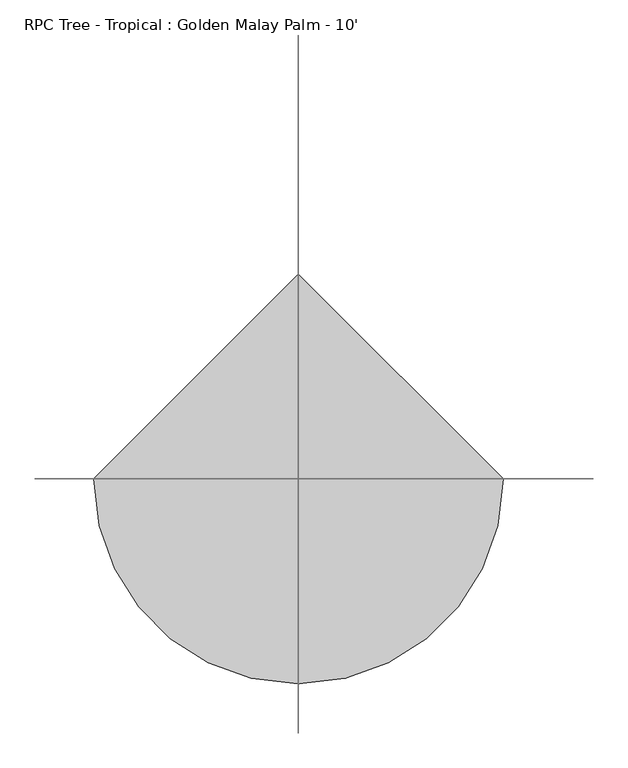
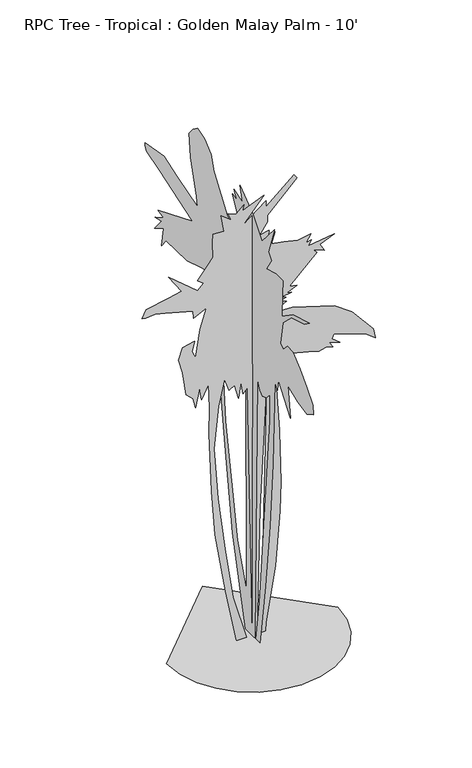
"""IFC4 building model written with IfcOpenShell, lengths in millimetres: geographic element geometry, RPC Tree - Tropical : Golden Malay Palm - 10'."""

from ifc_helpers import new_model, si_unit, origin, place, context, project, spatial, triangles, source, transform, mapped, element, save


def rpc_tree_tropical_golden_malay_palm_10_e9996539(model_context):
    return source(origin(), model_context, "Body", "Tessellation", [
        triangles([(-545.0582637, 0.0, 0.0), (-530.6500952, -124.8915047, 0.0), (-489.6100857, -239.5832322, 0.0), (-425.2296041, -340.7915895, 0.0), (-340.7915895, -425.2296041, 0.0), (-239.5832322, -489.6100857, 0.0), (-124.8912957, -530.6500952, 0.0), (2.38e-05, -545.0582637, 0.0), (124.8915047, -530.6500952, 0.0), (239.5832322, -489.6100857, 0.0), (340.7915895, -425.2296041, 0.0), (425.2296041, -340.7915895, 0.0), (489.6100857, -239.5832322, 0.0), (530.6500952, -124.8912957, 0.0), (545.0582637, 4.77e-05, 0.0), (-7.15e-05, 545.0582637, 0.0), (265.6838375, -8.79e-05, 3006.4903244), (285.0301493, -8.18e-05, 2977.4708748), (98.0157832, -5.84e-05, 2793.6806396), (98.0157832, -5.03e-05, 2748.5534523), (46.4256682, -3.97e-05, 2674.3855957), (107.6887302, -3.89e-05, 2687.276088), (104.4646265, -3.21e-05, 2648.5833916), (146.3815901, -3.29e-05, 2664.7123489), (123.8107385, -2.08e-05, 2590.5442017), (201.1958043, -1.45e-05, 2577.6537094), (291.4796285, -5.9e-06, 2555.0902611), (375.3122658, -4.6e-06, 2571.1979988), (343.0691031, 2.5e-06, 2522.8323463), (378.5359426, 3.1e-06, 2529.2880569), (359.1917381, 7.9e-06, 2497.0513618), (523.6333723, 1.22e-05, 2519.6148102), (430.1275609, 1.44e-05, 2480.9221138), (459.1470469, 2.5e-05, 2429.3390705), (388.2112241, 1.63e-05, 2458.3586655), (410.781249, 2.2e-05, 2432.5564613), (236.6643515, 4.32e-05, 2264.8953289), (285.0301493, 4.74e-05, 2255.2222275), (220.5417164, 4.87e-05, 2229.4200233), (249.5611842, 5.13e-05, 2222.985387), (188.2985537, 5e-05, 2213.3122856), (214.0943447, 5.36e-05, 2200.4005737), (172.1763365, 5.38e-05, 2187.5100815), (217.3180215, 5.89e-05, 2171.3811241), (117.3621042, 6.25e-05, 2123.0153263), (256.0106634, 7.01e-05, 2119.7979355), (523.6333723, 9.87e-05, 2035.961047), (633.2639626, 0.0001186, 1955.3521591), (771.9118223, 0.0001545, 1794.132058), (784.8087095, 0.0001672, 1726.419912), (729.9955582, 0.0001564, 1771.5620693), (520.4096955, 0.0001319, 1848.9473167), (507.5128447, 0.0001365, 1819.9278671), (559.1023192, 0.0001466, 1778.0094955), (491.3902096, 0.0001397, 1797.3556984), (513.9601982, 0.0001472, 1761.8889679), (468.8201846, 0.0001426, 1774.7857098), (423.6780636, 0.000142, 1765.1126083), (359.1917381, 0.0001359, 1781.2351707), (249.5611842, 0.0001251, 1810.2547657), (139.9327468, 0.0001121, 1852.1711025), (172.1763365, 0.0002094, 1316.9235409), (181.8497104, 0.0002716, 971.9134226), (175.400849, 0.0003059, 778.4502314), (149.6056938, 0.0003692, 417.3196218), (88.3424093, 0.0004301, 59.413947), (85.1180966, 0.0004411, 0.0034137), (46.4256682, 0.0004396, 5.62e-05), (72.220619, 0.0003162, 691.3939173), (98.0157832, 0.0001198, 1797.3556984), (49.6499854, 0.0002886, 839.7150238), (30.303451, 0.0004381, 0.0034157), (1.2840518, 0.0004366, 0.0034168), (-30.9596178, 0.0001346, 1678.0541142), (-59.9790969, 0.0001389, 1645.8110241), (-72.8765746, 0.0001232, 1729.6436977), (-85.7742612, 0.000141, 1626.4646759), (-111.5694254, 0.0001224, 1723.1962715), (-147.0375457, 0.0001247, 1700.6241028), (-176.0570226, 0.0001082, 1784.4589565), (-214.7505183, 0.0001362, 1616.7915745), (-243.7678787, 0.0001838, 1342.7193501), (-217.9741951, 0.0002468, 997.7092318), (-172.8324919, 0.0003125, 643.0281195), (-121.2423815, 0.0003762, 301.2416961), (-37.4084611, 0.0004339, 0.0067771), (-98.6717388, 0.0004315, 0.0034206), (-169.6081793, 0.000364, 356.0569731), (-237.320507, 0.0002879, 762.3297037), (-259.8905138, 0.0002331, 1062.1976646), (-276.0131488, 0.0001625, 1452.3478329), (-272.7873646, 0.0001316, 1626.4646759), (-279.2368438, 0.0001024, 1787.682597), (-321.1531443, 0.0001164, 1697.4004623), (-334.0521026, 0.0001008, 1781.2351707), (-359.8479117, 0.0001214, 1658.707766), (-375.9684394, 0.000109, 1723.1962715), (-421.1105604, 9.93e-05, 1765.1126083), (-443.680549, 6.99e-05, 1923.106889), (-469.4763582, 5.18e-05, 2016.6148441), (-443.680549, 3.99e-05, 2090.774271), (-366.2952653, 4.09e-05, 2106.8968334), (-382.4179367, 5.16e-05, 2042.4084732), (-359.8479117, 6.14e-05, 1994.0447102), (-330.8263184, 3.06e-05, 2174.5983696), (-292.1336765, 8.9e-06, 2306.8054161), (-372.7447626, 1.24e-05, 2264.8953289), (-375.9684394, 3.5e-06, 2313.2611267), (-553.3089955, -1.41e-05, 2361.6269245), (-617.7974648, -2.02e-05, 2377.7348076), (-679.0600771, -2.22e-05, 2371.3001713), (-701.6322458, -2.45e-05, 2377.7348076), (-675.8364367, -3.18e-05, 2426.1006054), (-533.9626837, -2.98e-05, 2455.1202003), (-450.1300464, -2.9e-05, 2474.4664032), (-533.9626837, -5.52e-05, 2597.0002029), (-346.9489534, -1.75e-05, 2439.0121719), (-311.4800065, -2.26e-05, 2477.7048683), (-346.9489534, -2.96e-05, 2506.7243179), (-285.6863229, -4.09e-05, 2587.3269562), (-250.2173578, -4.72e-05, 2632.4753632), (-253.4431602, -6.46e-05, 2729.2069588), (-250.2173578, -7.49e-05, 2787.2461487), (-179.2811354, -7.01e-05, 2780.7901474), (-198.6276652, -9.13e-05, 2893.6507004), (-134.13985, -7.88e-05, 2842.0465828), (-153.4863799, -8.84e-05, 2890.4122353), (-101.8960605, -8.18e-05, 2867.8487869), (-53.5304671, -8.8e-05, 2916.2144394), (-63.2034141, -8.15e-05, 2877.521743), (75.4451496, -8.49e-05, 2935.5609329), (-63.2034141, -6.37e-05, 2777.5729019), (88.3424093, -7.67e-05, 2893.6507004), (88.3424093, -6.92e-05, 2851.7195389), (3e-06, 92.9512395, 1743.2008644), (2.2e-06, 115.5032514, 1678.7654079), (-7.6e-06, 150.9419404, 1865.6266766), (-1.29e-05, 176.7159395, 1942.9463757), (-1.56e-05, 215.3770426, 1878.5129539), (-2.06e-05, 273.3673256, 1814.0773521), (-2.73e-05, 337.8028547, 1781.8617313), (-6.5e-06, 292.6988309, 1263.1644676), (3.07e-05, 160.607475, 544.7195852), (5.05e-05, 63.9556756, 264.4307708), (4.2e-06, 70.3992322, 1794.7480087), (-1.96e-05, 601.9838588, 3047.9979652), (-1e-05, 527.8836216, 3022.2169807), (7e-07, 453.7834208, 2961.0029846), (6.7e-06, 424.789333, 2874.0292236), (1.99e-05, 344.2459934, 2754.8187675), (3.13e-05, 273.3673256, 2654.9545143), (4.04e-05, 205.711299, 2619.5002831), (4.76e-05, 131.6119248, 2674.2794975), (3.24e-05, 218.5986119, 2838.596212), (3.89e-05, 167.0506137, 2825.7057198), (3.31e-05, 202.4895116, 2877.2467598), (4.55e-05, 105.8379257, 2848.2482391), (3.91e-05, 134.8332761, 2948.133712), (5.96e-05, -10.143928, 2838.596212), (7.48e-05, -106.795716, 2716.1685104), (8.65e-05, -245.3299745, 2877.2467598), (8.4e-05, -177.67353, 2690.3875259), (8.95e-05, -213.1122099, 2648.498513), (8.52e-05, -155.121509, 2561.524752), (9.7e-05, -261.437803, 2590.5232727), (0.0001062, -338.7595914, 2590.5232727), (0.0001082, -332.3164527, 2497.0935104), (0.0001124, -329.0948833, 2345.6672882), (0.0001241, -448.2991261, 2429.4238037), (0.000144, -628.715185, 2480.9645531), (0.000139, -577.168077, 2442.314296), (0.0001234, -435.4107413, 2400.4254284), (0.0001146, -338.7595914, 2310.2132023), (0.0001158, -309.7633962, 2152.3523438), (0.0001202, -341.9811607, 2133.0270699), (0.0001242, -387.0851664, 2181.3505737), (0.0001316, -448.2991261, 2178.1333282), (0.0001431, -528.8403583, 2113.6977264), (0.0001543, -602.9405954, 2033.156567), (0.0001647, -670.5976576, 1955.8346878), (0.0001673, -677.0407963, 1894.620837), (0.0001597, -602.9405954, 1852.7383644), (0.0001471, -503.0678398, 1875.2913483), (0.0001331, -396.7498744, 1920.3954266), (0.0001419, -419.3029309, 1714.2046692), (0.0001213, -290.4339983, 1891.3992313), (0.000122, -277.547739, 1817.3011379), (0.0001177, -251.7731132, 1855.9598248), (0.0001318, -229.2200385, 1292.1586281), (0.0001411, -197.0037636, 854.0046312), (0.0001482, -148.6779616, 422.2937731), (0.0001534, -87.4652644, 0.0055176), (0.000148, -42.3610362, 0.0055189), (0.0001443, -77.8001476, 267.652322), (0.0001199, -197.0037636, 1562.7848419), (0.0001147, -197.0037636, 1739.9792587), (0.0001114, -158.3430784, 1694.8753258), (0.0001065, -113.2390546, 1678.7654079), (0.0001024, -84.2434952, 1701.3183918), (9.75e-05, -58.4697051, 1762.5302078), (0.0001468, -32.695706, 0.0088781), (0.0001343, 73.6210059, 0.0055224), (0.0001006, 215.3770426, 560.8273956), (7.43e-05, 302.3635208, 1095.6346498), (4.55e-05, 386.1284297, 1727.0909466), (4.2e-05, 386.1284297, 1846.295153), (3.81e-05, 428.0109023, 1807.6342861), (3.77e-05, 389.349999, 1978.3856369), (3.3e-05, 424.789333, 1991.2740944), (3.2e-05, 405.4578094, 2104.0330547), (2.83e-05, 440.8971434, 2084.7037113), (2.46e-05, 453.7834208, 2158.8080544), (1.3e-05, 556.8798168, 2136.2444607), (-4.7e-06, 717.9643885, 2084.7037113), (-3.21e-05, 949.9297354, 2078.2605), (-3.61e-05, 998.2553467, 2017.0465038), (-3.71e-05, 975.7022902, 2142.7003166), (-4.74e-05, 1075.5771532, 2087.9251717), (-4.1e-05, 998.2553467, 2181.3505737), (-4.9e-05, 1069.1340145, 2165.242836), (-3.97e-05, 978.9259306, 2216.7835854), (-4.71e-05, 1036.9162136, 2232.9125427), (-6.8e-06, 659.9741055, 2387.5349361), (-5.42e-05, 1027.2515419, 2509.9627831), (-7.19e-05, 1165.7851645, 2548.6342598), (-7.47e-05, 1181.8929749, 2577.6327805), (-7.53e-05, 1181.8929749, 2596.9577637), (-5.14e-05, 972.4806845, 2632.3907753), (-3.19e-05, 821.0608572, 2584.0672714), (-4.1e-06, 605.2054281, 2516.4187843), (-6.9e-06, 611.6485668, 2584.0672714), (-2.16e-05, 679.305629, 2806.3595169), (-2.8e-05, 695.4134394, 2957.7857391), (-2.46e-05, 653.5309668, 3009.3477081), (4.12e-05, 25.2952084, 1846.295153), (9.49e-05, 2.7429654, 132.3394149), (4.6e-05, -10.1438644, 1826.9658096)], [[15, 16, 1], [14, 15, 1], [14, 1, 2], [13, 14, 2], [13, 2, 3], [13, 3, 4], [12, 13, 4], [11, 12, 4], [11, 4, 5], [11, 5, 6], [11, 6, 7], [11, 7, 8], [11, 8, 9], [11, 9, 10], [31, 32, 33], [115, 116, 117], [39, 40, 41], [76, 77, 78], [53, 54, 55], [95, 96, 97], [130, 131, 132], [128, 129, 130], [37, 38, 39], [93, 94, 95], [33, 34, 35], [49, 50, 51], [31, 33, 35], [55, 56, 57], [124, 125, 126], [41, 42, 43], [126, 127, 128], [27, 28, 29], [43, 44, 45], [29, 30, 31], [74, 75, 76], [23, 24, 25], [132, 133, 134], [101, 102, 103], [106, 107, 108], [100, 101, 103], [21, 22, 23], [128, 130, 132], [126, 128, 132], [78, 79, 80], [85, 86, 87], [85, 87, 88], [84, 85, 88], [84, 88, 89], [83, 84, 89], [83, 89, 90], [82, 83, 90], [82, 90, 91], [81, 82, 91], [81, 91, 92], [48, 49, 51], [48, 51, 52], [111, 112, 113], [47, 48, 52], [110, 111, 113], [110, 113, 114], [109, 110, 114], [134, 17, 18], [134, 18, 19], [132, 134, 19], [95, 97, 98], [67, 68, 69], [66, 67, 69], [65, 66, 69], [64, 65, 69], [64, 69, 70], [63, 64, 70], [62, 63, 70], [61, 62, 70], [124, 126, 132], [132, 19, 20], [132, 20, 21], [95, 98, 99], [122, 123, 124], [99, 100, 103], [99, 103, 104], [72, 73, 74], [71, 72, 74], [70, 71, 74], [70, 74, 76], [118, 119, 120], [95, 99, 104], [93, 95, 104], [35, 36, 37], [80, 81, 92], [80, 92, 93], [108, 109, 114], [108, 114, 115], [108, 115, 117], [106, 108, 117], [31, 35, 37], [46, 47, 52], [46, 52, 53], [46, 53, 55], [46, 55, 57], [46, 57, 58], [46, 58, 59], [46, 59, 60], [46, 60, 61], [45, 46, 61], [80, 93, 104], [106, 117, 118], [29, 31, 37], [27, 29, 37], [26, 27, 37], [25, 26, 37], [121, 122, 124], [121, 124, 132], [121, 132, 21], [76, 78, 80], [80, 104, 105], [70, 76, 80], [70, 80, 105], [61, 70, 105], [45, 61, 105], [45, 105, 106], [43, 45, 106], [41, 43, 106], [41, 106, 118], [41, 118, 120], [41, 120, 121], [41, 121, 21], [41, 21, 23], [41, 23, 25], [41, 25, 37], [41, 37, 39], [235, 144, 145], [144, 235, 236], [219, 220, 221], [160, 161, 162], [169, 170, 171], [169, 171, 172], [217, 218, 219], [215, 216, 217], [184, 185, 186], [135, 136, 137], [168, 169, 172], [168, 172, 173], [206, 207, 208], [157, 158, 159], [221, 222, 223], [155, 156, 157], [186, 187, 188], [145, 135, 146], [145, 146, 147], [145, 147, 148], [145, 148, 149], [145, 149, 150], [145, 150, 151], [153, 154, 155], [145, 151, 152], [235, 145, 152], [210, 211, 212], [192, 193, 194], [191, 192, 194], [191, 194, 195], [190, 191, 195], [189, 190, 195], [188, 189, 195], [188, 195, 196], [165, 166, 167], [153, 155, 157], [153, 157, 159], [153, 159, 160], [226, 227, 228], [225, 226, 228], [224, 225, 228], [223, 224, 228], [223, 228, 229], [223, 229, 230], [208, 209, 210], [201, 202, 203], [162, 163, 164], [160, 162, 164], [153, 160, 164], [214, 215, 217], [164, 165, 167], [164, 167, 168], [235, 152, 153], [235, 153, 164], [235, 164, 168], [235, 168, 173], [235, 173, 174], [237, 235, 174], [237, 174, 175], [180, 181, 182], [179, 180, 182], [179, 182, 183], [179, 183, 184], [178, 179, 184], [177, 178, 184], [176, 177, 184], [175, 176, 184], [237, 175, 184], [237, 184, 186], [237, 186, 188], [237, 188, 196], [237, 196, 197], [217, 219, 221], [214, 217, 221], [214, 221, 223], [213, 214, 223], [212, 213, 223], [212, 223, 230], [197, 198, 199], [197, 199, 200], [237, 197, 200], [236, 237, 200], [236, 200, 201], [236, 201, 203], [144, 236, 203], [143, 144, 203], [142, 143, 203], [142, 203, 204], [142, 204, 205], [141, 142, 205], [141, 205, 206], [140, 141, 206], [140, 206, 208], [139, 140, 208], [138, 139, 208], [138, 208, 210], [232, 233, 234], [232, 234, 146], [231, 232, 146], [210, 212, 230], [138, 210, 230], [138, 230, 231], [138, 231, 146], [138, 146, 135], [138, 135, 137]], closed=False),
    ])


if __name__ == "__main__":
    model = new_model("IFC4")
    model_context = context("Model", 3, world=origin())
    ifc_project = project(units=[si_unit("LENGTHUNIT", "METRE", prefix="MILLI")], contexts=[model_context])
    site = spatial("IfcSite", under=ifc_project)
    building = spatial("IfcBuilding", under=site)
    placement = place(None, origin())
    rpc_tree_tropical_golden_malay_palm_10_shape = rpc_tree_tropical_golden_malay_palm_10_e9996539(model_context)
    element("IfcGeographicElement", 1, ObjectType="RPC Tree - Tropical : Golden Malay Palm - 10'", at=placement, inside=building, context=model_context, shape_type="MappedRepresentation", body=[
        mapped(rpc_tree_tropical_golden_malay_palm_10_shape, transform((0.0, 0.0, 0.0), x_axis=(1.0, 0.0, 0.0), y_axis=(0.0, 1.0, 0.0), z_axis=(0.0, 0.0, 1.0))),
    ])
    save(model, "model.ifc")

# Revit data of these elements
# Type "RPC Tree - Tropical : Golden Malay Palm - 10'"
#   built-in parameter 1005195 = "RPC-16-FXGL-UL7X-PH44-0000-ST1L-LVER-AU"
#   Type Comments = "Golden Malay Palm"
#   Assembly Code = "G2050500"
#   Height = 10' - 0"
#   Plan Symbol = element 497571
#   Default Elevation = 0
